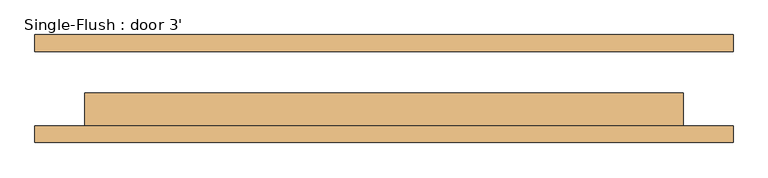
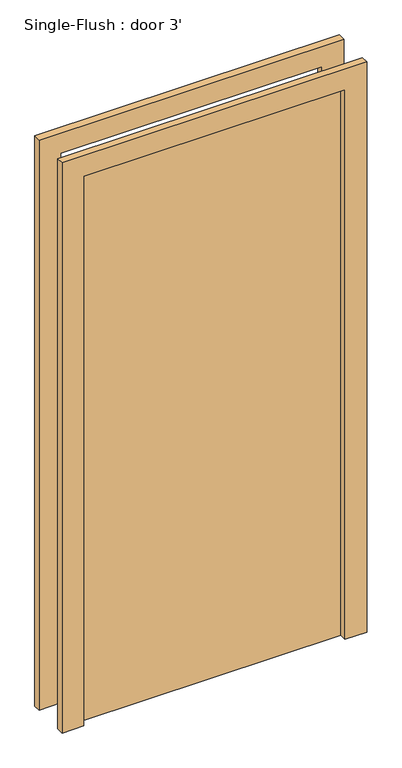
"""IFC4 building model written with IfcOpenShell, lengths in millimetres: door geometry, Single-Flush : door 3'."""

from ifc_helpers import new_model, si_unit, frame, origin, origin_with_axes, place, context, project, spatial, polyline, outline, extrude, source, transform, mapped, element, save


def single_flush_door_3_5e62189b(model_context):
    return source(origin(), model_context, "Body", "SweptSolid", [
        extrude(outline(polyline([(2108.2, -533.4), (0.0, -533.4), (0.0, -457.2), (2032.0, -457.2), (2032.0, 457.2), (0.0, 457.2), (0.0, 533.4), (2108.2, 533.4), (2108.2, -533.4)])), frame((0.0, -82.55, 0.0), z_axis=(0.0, 1.0, 0.0), x_axis=(0.0, 0.0, 1.0)), (0.0, 0.0, 1.0), 25.4),
        extrude(outline(polyline([(2108.2, 533.4), (2108.2, -533.4), (0.0, -533.4), (0.0, -457.2), (2032.0, -457.2), (2032.0, 457.2), (0.0, 457.2), (0.0, 533.4), (2108.2, 533.4)])), frame((0.0, 57.15, 0.0), z_axis=(0.0, 1.0, 0.0), x_axis=(0.0, 0.0, 1.0)), (0.0, 0.0, 1.0), 25.4),
        extrude(outline(polyline([(457.2, -6.35), (457.2, -57.15), (-457.2, -57.15), (-457.2, -6.35), (457.2, -6.35)])), origin_with_axes(), (0.0, 0.0, 1.0), 2032.0),
    ])


if __name__ == "__main__":
    model = new_model("IFC4")
    model_context = context("Model", 3, world=origin())
    ifc_project = project(units=[si_unit("LENGTHUNIT", "METRE", prefix="MILLI")], contexts=[model_context])
    site = spatial("IfcSite", under=ifc_project)
    building = spatial("IfcBuilding", under=site)
    placement = place(None, origin())
    single_flush_door_3_shape = single_flush_door_3_5e62189b(model_context)
    element("IfcDoor", 1, ObjectType="Single-Flush : door 3'", at=placement, inside=building, context=model_context, shape_type="MappedRepresentation", body=[
        mapped(single_flush_door_3_shape, transform((0.0, 0.0, 0.0), x_axis=(1.0, 0.0, 0.0), y_axis=(0.0, 1.0, 0.0), z_axis=(0.0, 0.0, 1.0))),
    ])
    save(model, "model.ifc")

# Revit data of these elements
# Type "Single-Flush : door 3'"
#   Type Mark = "9"
#   Construction Type Id = "MDOOR"
#   Assembly Code = "C1020"
#   Analytic Construction = "Metal"
#   Thickness = 0' - 2"
#   Heat Transfer Coefficient (U) = 0.651978 BTU/(h·ft²·°F)
#   Height = 6' - 8"
#   Trim Projection Ext = 0' - 1"
#   Trim Projection Int = 0' - 1"
#   Trim Width = 0' - 3"
#   Width = 3' - 0"
#   Define Thermal Properties by = 1
#   Door Material = Door - Panel
#   Frame Material = Door - Frame
#   Visual Light Transmittance = 0
#   Solar Heat Gain Coefficient = 0
#   Function = (empty or 0)
#   Wall Closure = (empty or 0)
# Element 1 (IfcDoor, "Single-Flush : door 3'")
#   Materials on its faces: "Door - Frame", "Door - Panel"
# Materials
#   "Door - Panel": class "Wood", colour RGB 210 159 95, transparency 0, Cost = 0
#   "Door - Frame": colour RGB 118 70 51, transparency 0, Cost = 0
